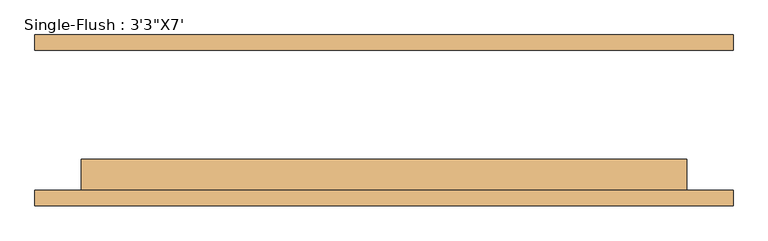
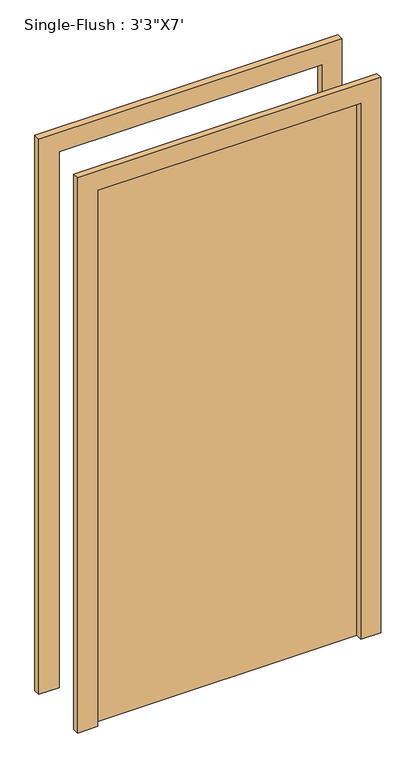
"""IFC4 building model written with IfcOpenShell, lengths in millimetres: door geometry."""

from ifc_helpers import new_model, si_unit, frame, origin, origin_with_axes, place, context, project, spatial, polyline, outline, extrude, source, transform, mapped, element, save


def door_49933fe7(model_context):
    return source(origin(), model_context, "Body", "SweptSolid", [
        extrude(outline(polyline([(2209.8, -571.5), (0.0, -571.5), (0.0, -495.3), (2133.6, -495.3), (2133.6, 495.3), (0.0, 495.3), (0.0, 571.5), (2209.8, 571.5), (2209.8, -571.5)])), frame((0.0, -139.7, 0.0), z_axis=(0.0, 1.0, 0.0), x_axis=(0.0, 0.0, 1.0)), (0.0, 0.0, 1.0), 25.4),
        extrude(outline(polyline([(2209.8, 571.5), (2209.8, -571.5), (0.0, -571.5), (0.0, -495.3), (2133.6, -495.3), (2133.6, 495.3), (0.0, 495.3), (0.0, 571.5), (2209.8, 571.5)])), frame((0.0, 114.3, 0.0), z_axis=(0.0, 1.0, 0.0), x_axis=(0.0, 0.0, 1.0)), (0.0, 0.0, 1.0), 25.4),
        extrude(outline(polyline([(495.3, -63.5), (495.3, -114.3), (-495.3, -114.3), (-495.3, -63.5), (495.3, -63.5)])), origin_with_axes(), (0.0, 0.0, 1.0), 2133.6),
    ])


if __name__ == "__main__":
    model = new_model("IFC4")
    model_context = context("Model", 3, world=origin())
    ifc_project = project(units=[si_unit("LENGTHUNIT", "METRE", prefix="MILLI")], contexts=[model_context])
    site = spatial("IfcSite", under=ifc_project)
    building = spatial("IfcBuilding", under=site)
    placement = place(None, origin())
    door_shape = door_49933fe7(model_context)
    element("IfcDoor", 1, ObjectType="Single-Flush : 3'3\"X7'", at=placement, inside=building, context=model_context, shape_type="MappedRepresentation", body=[
        mapped(door_shape, transform((0.0, 0.0, 0.0), x_axis=(1.0, 0.0, 0.0), y_axis=(0.0, 1.0, 0.0), z_axis=(0.0, 0.0, 1.0))),
    ])
    save(model, "model.ifc")

# Revit data of these elements
# Type "Single-Flush : 3'3\"X7'"
#   Type Mark = "11"
#   Construction Type Id = "MDOOR"
#   Assembly Code = "C1020"
#   Analytic Construction = "Metal"
#   Thickness = 0' - 2"
#   Heat Transfer Coefficient (U) = 0.651978 BTU/(h·ft²·°F)
#   Height = 7' - 0"
#   Trim Projection Ext = 0' - 1"
#   Trim Projection Int = 0' - 1"
#   Trim Width = 0' - 3"
#   Width = 3' - 3"
#   Define Thermal Properties by = 1
#   Door Material = Door - Panel
#   Frame Material = Door - Frame
#   Visual Light Transmittance = 0
#   Solar Heat Gain Coefficient = 0
#   Function = (empty or 0)
#   Wall Closure = (empty or 0)
# Element 1 (IfcDoor, "Single-Flush : 3'3\"X7'")
#   Materials on its faces: "Door - Frame", "Door - Panel"
# Materials
#   "Door - Panel": class "Wood", colour RGB 210 159 95, transparency 0, Cost = 0
#   "Door - Frame": colour RGB 118 70 51, transparency 0, Cost = 0
